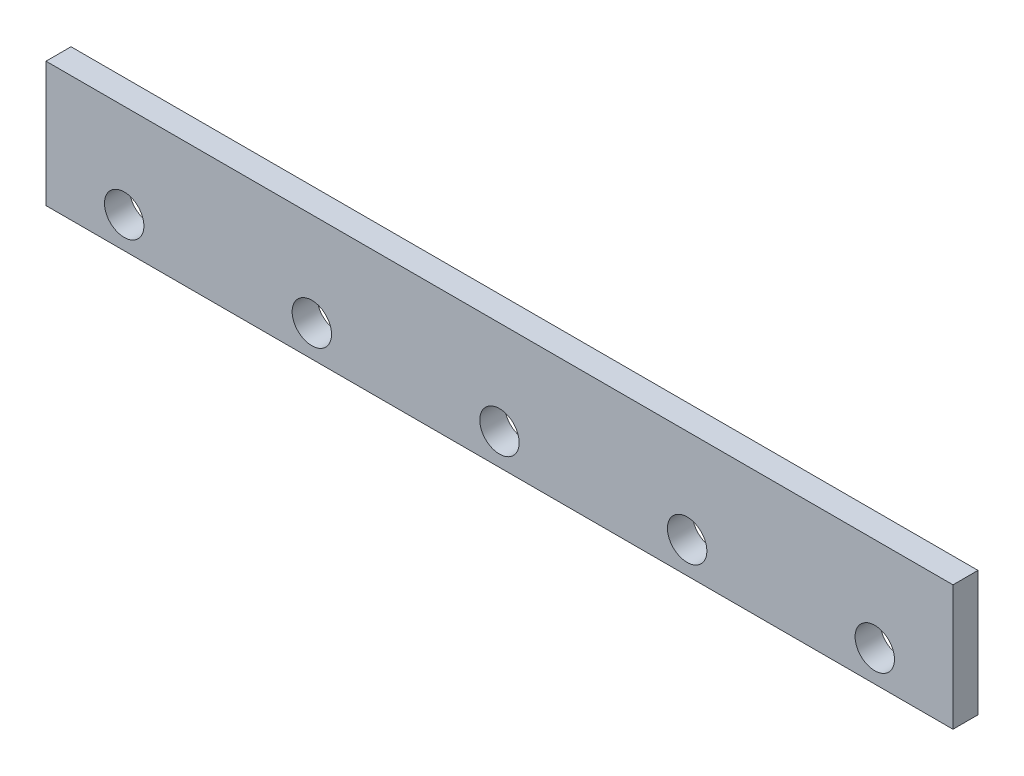
from build123d import *

# Parameters (mm, degrees)
BAR_PROFILE_SKETCH_W      = 580
BAR_PROFILE_SKETCH_H      = 80
FLAT_BAR_580X80X16_DEPTH  = 16
HOLE_ROW_SKETCH_R         = 12.6
THROUGH_HOLES_5X_20_DEPTH = 16


with BuildPart() as part:
    # Bar Profile Sketch → Flat Bar 580x80x16 (new body)
    with BuildSketch(Plane.XY):
        Rectangle(BAR_PROFILE_SKETCH_W, BAR_PROFILE_SKETCH_H)
    extrude(amount=FLAT_BAR_580X80X16_DEPTH)

    # Hole Row Sketch → Through Holes 5xØ20 (cut)
    with BuildSketch(Plane.XY.offset(16)):
        with Locations((-240, -20)):
            Circle(HOLE_ROW_SKETCH_R)
        with Locations((-120, -20)):
            Circle(HOLE_ROW_SKETCH_R)
        with Locations((0, -20)):
            Circle(HOLE_ROW_SKETCH_R)
        with Locations((120, -20)):
            Circle(HOLE_ROW_SKETCH_R)
        with Locations((240, -20)):
            Circle(HOLE_ROW_SKETCH_R)
    extrude(amount=-THROUGH_HOLES_5X_20_DEPTH, mode=Mode.SUBTRACT)


solid = part.part
